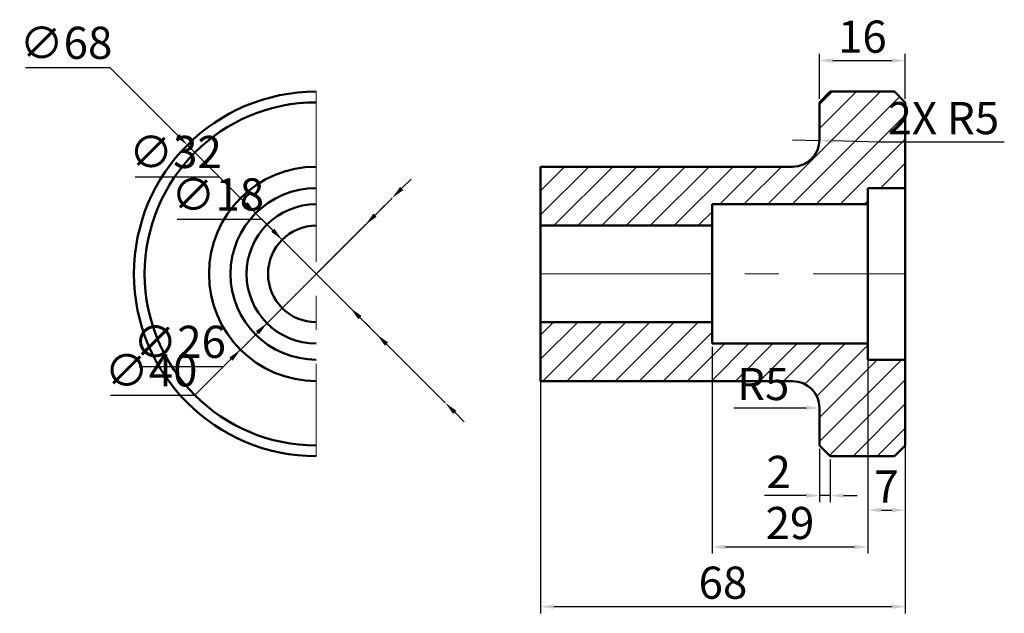
# Model space of a CAD drawing. Units: millimetres. Extents: x 43 to 227, y -15 to 96.
import ezdxf

# ---------------------------------------------------------------- set-up
doc = ezdxf.new("R2010")
doc.units = ezdxf.units.MM
doc.linetypes.add('CENTER', pattern=[50.8, 31.75, -6.35, 6.35, -6.35])
for name, color, linetype, lineweight in [('M-CNTR', 1, 'CENTER', 18), ('M-DIMS', 2, 'Continuous', 25), ('M-HATC', 8, 'Continuous', 18), ('M-OUTL', 7, 'Continuous', 50)]:
    doc.layers.add(name, color=color, linetype=linetype, lineweight=lineweight)
doc.styles.get("Standard").update_dxf_attribs({"font": 'arial.ttf'})
doc.dimstyles.new('ISO-25', dxfattribs={"dimtxt": 6, "dimasz": 2.5, "dimexe": 1.25, "dimexo": 0.625, "dimtad": 1, "dimtoh": 1, "dimdec": 0, "dimtxsty": 'Standard', "dimcen": 2.5, "dimadec": 0, "dimazin": 0, "dimtfac": 1, "dimtdec": 0, "dimtmove": 0, "dimatfit": 3, "dimfxl": 1, "dimarcsym": 0})

# ---------------------------------------------------------------- blocks, each defined once
blk = doc.blocks.new('*D1')
at = {"layer": 'Defpoints', "color": 0, "transparency": 16777216}
for p in [(172.49, 35.65), (201.49, 35.65), (201.49, -2.28)]:
    blk.add_point(p, dxfattribs=at)
at = {"layer": 'M-DIMS', "color": 0, "lineweight": -2, "transparency": 16777216}
for p, q in [((172.49, 35.03), (172.49, -3.53)), ((201.49, 35.03), (201.49, -3.53)), ((174.99, -2.28), (198.99, -2.28))]:
    blk.add_line(p, q, dxfattribs=at)
at = {"layer": 'M-DIMS', "color": 0, "transparency": 16777216}
for points in [[(174.99, -1.87), (174.99, -2.7), (172.49, -2.28)], [(198.99, -1.87), (198.99, -2.7), (201.49, -2.28)]]:
    blk.add_solid(points, dxfattribs=at)
at = {"layer": 'M-DIMS', "color": 0, "transparency": 16777216, "insert": (186.99, 1.41), "char_height": 6, "attachment_point": 5}
blk.add_mtext('29', dxfattribs=at)
blk = doc.blocks.new('*D2')
at = {"layer": 'Defpoints', "color": 0, "transparency": 16777216}
for p in [(140.49, 48.65), (208.49, 48.65), (208.49, -13.41)]:
    blk.add_point(p, dxfattribs=at)
at = {"layer": 'M-DIMS', "color": 0, "lineweight": -2, "transparency": 16777216}
for p, q in [((140.49, 48.03), (140.49, -14.66)), ((208.49, 48.03), (208.49, -14.66)), ((142.99, -13.41), (205.99, -13.41))]:
    blk.add_line(p, q, dxfattribs=at)
at = {"layer": 'M-DIMS', "color": 0, "transparency": 16777216}
for points in [[(142.99, -12.99), (142.99, -13.82), (140.49, -13.41)], [(205.99, -12.99), (205.99, -13.82), (208.49, -13.41)]]:
    blk.add_solid(points, dxfattribs=at)
at = {"layer": 'M-DIMS', "color": 0, "transparency": 16777216, "insert": (174.49, -9.72), "char_height": 6, "attachment_point": 5}
blk.add_mtext('68', dxfattribs=at)
blk = doc.blocks.new('*D3')
at = {"layer": 'Defpoints', "color": 0, "transparency": 16777216}
for p in [(208.49, 88.44), (192.49, 80.65), (208.49, 80.65)]:
    blk.add_point(p, dxfattribs=at)
at = {"layer": 'M-DIMS', "color": 0, "lineweight": -2, "transparency": 16777216}
for p, q in [((192.49, 81.28), (192.49, 89.69)), ((194.99, 88.44), (205.99, 88.44)), ((208.49, 81.28), (208.49, 89.69))]:
    blk.add_line(p, q, dxfattribs=at)
at = {"layer": 'M-DIMS', "color": 0, "transparency": 16777216}
for points in [[(194.99, 88.86), (194.99, 88.03), (192.49, 88.44)], [(205.99, 88.86), (205.99, 88.03), (208.49, 88.44)]]:
    blk.add_solid(points, dxfattribs=at)
at = {"layer": 'M-DIMS', "color": 0, "transparency": 16777216, "insert": (200.49, 92.13), "char_height": 6, "attachment_point": 5}
blk.add_mtext('16', dxfattribs=at)
blk = doc.blocks.new('*D4')
at = {"layer": 'Defpoints', "color": 0, "transparency": 16777216}
for p in [(187.49, 23.65), (192.49, 23.65)]:
    blk.add_point(p, dxfattribs=at)
at = {"layer": 'M-DIMS', "color": 0, "lineweight": -2, "transparency": 16777216}
blk.add_line((176.52, 23.65), (189.99, 23.65), dxfattribs=at)
at = {"layer": 'M-DIMS', "color": 0, "transparency": 16777216}
blk.add_solid([(189.99, 24.07), (189.99, 23.24), (192.49, 23.65)], dxfattribs=at)
at = {"layer": 'M-DIMS', "color": 0, "transparency": 16777216, "insert": (182, 27.33), "char_height": 6, "attachment_point": 5}
blk.add_mtext('R5', dxfattribs=at)
blk = doc.blocks.new('*D5')
at = {"layer": 'Defpoints', "color": 0, "transparency": 16777216}
for p in [(201.49, 32.65), (208.49, 32.65), (208.49, 4.6)]:
    blk.add_point(p, dxfattribs=at)
at = {"layer": 'M-DIMS', "color": 0, "lineweight": -2, "transparency": 16777216}
for p, q in [((201.49, 32.03), (201.49, 3.35)), ((208.49, 32.03), (208.49, 3.35)), ((203.99, 4.6), (205.99, 4.6))]:
    blk.add_line(p, q, dxfattribs=at)
at = {"layer": 'M-DIMS', "color": 0, "transparency": 16777216}
for points in [[(203.99, 5.01), (203.99, 4.18), (201.49, 4.6)], [(205.99, 5.01), (205.99, 4.18), (208.49, 4.6)]]:
    blk.add_solid(points, dxfattribs=at)
at = {"layer": 'M-DIMS', "color": 0, "transparency": 16777216, "insert": (204.99, 8.22), "char_height": 6, "attachment_point": 5}
blk.add_mtext('7', dxfattribs=at)
blk = doc.blocks.new('*D6')
at = {"layer": 'Defpoints', "color": 0, "transparency": 16777216}
for p in [(192.49, 16.65), (194.49, 14.65), (192.49, 7.3)]:
    blk.add_point(p, dxfattribs=at)
at = {"layer": 'M-DIMS', "color": 0, "lineweight": -2, "transparency": 16777216}
for p, q in [((192.49, 16.03), (192.49, 6.05)), ((194.49, 14.03), (194.49, 6.05)), ((189.99, 7.3), (182.26, 7.3)), ((194.49, 7.3), (192.49, 7.3)), ((196.99, 7.3), (199.49, 7.3))]:
    blk.add_line(p, q, dxfattribs=at)
at = {"layer": 'M-DIMS', "color": 0, "transparency": 16777216}
for points in [[(189.99, 7.72), (189.99, 6.89), (192.49, 7.3)], [(196.99, 7.72), (196.99, 6.89), (194.49, 7.3)]]:
    blk.add_solid(points, dxfattribs=at)
at = {"layer": 'M-DIMS', "color": 0, "transparency": 16777216, "insert": (184.88, 10.94), "char_height": 6, "attachment_point": 5}
blk.add_mtext('2', dxfattribs=at)
blk = doc.blocks.new('*D7')
at = {"layer": 'Defpoints', "color": 0, "transparency": 16777216}
for p in [(74.64, 72.69), (122.72, 24.61)]:
    blk.add_point(p, dxfattribs=at)
at = {"layer": 'M-DIMS', "color": 0, "lineweight": -2, "transparency": 16777216}
for p, q in [((44.45, 87.12), (60.21, 87.12)), ((60.21, 87.12), (72.87, 74.46)), ((122.72, 24.61), (74.64, 72.69)), ((124.49, 22.85), (126.26, 21.08))]:
    blk.add_line(p, q, dxfattribs=at)
at = {"layer": 'M-DIMS', "color": 0, "transparency": 16777216}
for points in [[(73.16, 74.76), (72.57, 74.17), (74.64, 72.69)], [(124.79, 23.14), (124.2, 22.55), (122.72, 24.61)]]:
    blk.add_solid(points, dxfattribs=at)
at = {"layer": 'M-DIMS', "color": 0, "transparency": 16777216, "insert": (52.02, 90.97), "char_height": 6, "attachment_point": 5}
blk.add_mtext('∅68', dxfattribs=at)
blk = doc.blocks.new('*D8')
at = {"layer": 'Defpoints', "color": 0, "transparency": 16777216}
for p in [(112.82, 62.8), (84.54, 34.51)]:
    blk.add_point(p, dxfattribs=at)
at = {"layer": 'M-DIMS', "color": 0, "lineweight": -2, "transparency": 16777216}
for p, q in [((114.59, 64.57), (116.36, 66.33)), ((112.82, 62.8), (84.54, 34.51)), ((76.06, 26.02), (82.77, 32.74)), ((60.33, 26.02), (76.06, 26.02))]:
    blk.add_line(p, q, dxfattribs=at)
at = {"layer": 'M-DIMS', "color": 0, "transparency": 16777216}
for points in [[(114.29, 64.86), (114.88, 64.27), (112.82, 62.8)], [(82.48, 33.04), (83.07, 32.45), (84.54, 34.51)]]:
    blk.add_solid(points, dxfattribs=at)
at = {"layer": 'M-DIMS', "color": 0, "transparency": 16777216, "insert": (67.88, 29.88), "char_height": 6, "attachment_point": 5}
blk.add_mtext('∅40', dxfattribs=at)
blk = doc.blocks.new('*D9')
at = {"layer": 'Defpoints', "color": 0, "transparency": 16777216}
for p in [(87.37, 59.97), (109.99, 37.34)]:
    blk.add_point(p, dxfattribs=at)
at = {"layer": 'M-DIMS', "color": 0, "lineweight": -2, "transparency": 16777216}
for p, q in [((64.9, 66.76), (80.58, 66.76)), ((80.58, 66.76), (85.6, 61.74)), ((109.99, 37.34), (87.37, 59.97)), ((111.76, 35.57), (113.53, 33.8))]:
    blk.add_line(p, q, dxfattribs=at)
at = {"layer": 'M-DIMS', "color": 0, "transparency": 16777216}
for points in [[(85.9, 62.03), (85.31, 61.44), (87.37, 59.97)], [(112.05, 35.86), (111.46, 35.28), (109.99, 37.34)]]:
    blk.add_solid(points, dxfattribs=at)
at = {"layer": 'M-DIMS', "color": 0, "transparency": 16777216, "insert": (72.43, 70.62), "char_height": 6, "attachment_point": 5}
blk.add_mtext('∅32', dxfattribs=at)
blk = doc.blocks.new('*D10')
at = {"layer": 'Defpoints', "color": 0, "transparency": 16777216}
for p in [(107.87, 57.85), (89.49, 39.46)]:
    blk.add_point(p, dxfattribs=at)
at = {"layer": 'M-DIMS', "color": 0, "lineweight": -2, "transparency": 16777216}
for p, q in [((109.64, 59.62), (111.41, 61.38)), ((107.87, 57.85), (89.49, 39.46)), ((81.39, 31.35), (87.72, 37.69)), ((65.64, 31.35), (81.39, 31.35))]:
    blk.add_line(p, q, dxfattribs=at)
at = {"layer": 'M-DIMS', "color": 0, "transparency": 16777216}
for points in [[(109.34, 59.91), (109.93, 59.32), (107.87, 57.85)], [(87.43, 37.99), (88.02, 37.4), (89.49, 39.46)]]:
    blk.add_solid(points, dxfattribs=at)
at = {"layer": 'M-DIMS', "color": 0, "transparency": 16777216, "insert": (73.2, 35.21), "char_height": 6, "attachment_point": 5}
blk.add_mtext('∅26', dxfattribs=at)
blk = doc.blocks.new('*D11')
at = {"layer": 'Defpoints', "color": 0, "transparency": 16777216}
for p in [(92.32, 55.02), (105.04, 42.29)]:
    blk.add_point(p, dxfattribs=at)
at = {"layer": 'M-DIMS', "color": 0, "lineweight": -2, "transparency": 16777216}
for p, q in [((72.74, 58.84), (88.5, 58.84)), ((88.5, 58.84), (90.55, 56.79)), ((105.04, 42.29), (92.32, 55.02)), ((106.81, 40.52), (108.58, 38.75))]:
    blk.add_line(p, q, dxfattribs=at)
at = {"layer": 'M-DIMS', "color": 0, "transparency": 16777216}
for points in [[(90.85, 57.08), (90.26, 56.49), (92.32, 55.02)], [(107.1, 40.81), (106.51, 40.22), (105.04, 42.29)]]:
    blk.add_solid(points, dxfattribs=at)
at = {"layer": 'M-DIMS', "color": 0, "transparency": 16777216, "insert": (80.31, 62.7), "char_height": 6, "attachment_point": 5}
blk.add_mtext('∅18', dxfattribs=at)
blk = doc.blocks.new('*D12')
at = {"layer": 'Defpoints', "color": 0, "transparency": 16777216}
for p in [(187.49, 73.65), (192.49, 73.53)]:
    blk.add_point(p, dxfattribs=at)
at = {"layer": 'M-DIMS', "color": 0, "lineweight": -2, "transparency": 16777216}
for p, q in [((187.49, 73.65), (192.49, 73.53)), ((203.61, 73.24), (194.99, 73.46)), ((226.95, 73.24), (203.61, 73.24))]:
    blk.add_line(p, q, dxfattribs=at)
at = {"layer": 'M-DIMS', "color": 0, "transparency": 16777216}
blk.add_solid([(195, 73.88), (194.98, 73.05), (192.49, 73.53)], dxfattribs=at)
at = {"layer": 'M-DIMS', "color": 0, "transparency": 16777216, "insert": (215.59, 76.93), "char_height": 6, "attachment_point": 5}
blk.add_mtext('2X R5', dxfattribs=at)

msp = doc.modelspace()

# ---------------------------------------------------------------- hatches: boundary and pattern name
at = {"layer": 'M-HATC'}
h = msp.add_hatch(dxfattribs=at)
h.set_pattern_fill('ANSI31', color=256)
h.paths.add_polyline_path([(201.49, 64.65), (208.49, 64.65), (208.49, 80.65), (206.49, 82.65), (194.49, 82.65), (192.49, 80.65), (192.49, 73.65, -0.414214), (187.49, 68.65), (140.49, 68.65), (140.49, 57.65), (172.49, 57.65), (172.49, 61.65), (201.49, 61.65)])
h.paths.add_polyline_path([(208.49, 32.65), (201.49, 32.65), (201.49, 35.65), (179.49, 35.65), (172.49, 35.65), (172.49, 39.65), (140.49, 39.65), (140.49, 28.65), (187.49, 28.65, -0.414214), (192.49, 23.65), (192.49, 16.65), (194.49, 14.65), (206.49, 14.65), (208.49, 16.65)])

# ---------------------------------------------------------------- linework, layer by layer
at = {"layer": 'M-CNTR'}
for p, q in [((98.68, 82.65), (98.68, 14.65)), ((140.49, 48.65), (208.49, 48.65))]:
    msp.add_line(p, q, dxfattribs=at)
at = {"layer": 'M-OUTL'}
for p, q in [((192.49, 80.65), (194.49, 82.65)), ((194.49, 82.65), (206.49, 82.65)), ((206.49, 82.65), (208.49, 80.65)), ((192.49, 73.65), (192.49, 80.65)), ((208.49, 80.65), (208.49, 16.65)), ((140.49, 48.65), (140.49, 68.65)), ((140.49, 48.65), (140.49, 68.65)), ((140.49, 68.65), (187.49, 68.65)), ((201.49, 64.65), (208.49, 64.65)), ((201.49, 64.65), (201.49, 32.65)), ((172.49, 61.65), (201.49, 61.65)), ((172.49, 48.65), (172.49, 61.65)), ((140.49, 57.65), (172.49, 57.65)), ((140.49, 48.65), (140.49, 28.65)), ((172.49, 48.65), (172.49, 35.65)), ((140.49, 39.65), (172.49, 39.65)), ((179.49, 35.65), (172.49, 35.65)), ((179.49, 35.65), (201.49, 35.65)), ((201.49, 32.65), (208.49, 32.65)), ((140.49, 28.65), (187.49, 28.65)), ((192.49, 23.65), (192.49, 16.65)), ((192.49, 16.65), (194.49, 14.65)), ((208.49, 16.65), (206.49, 14.65)), ((206.49, 14.65), (194.49, 14.65))]:
    msp.add_line(p, q, dxfattribs=at)
for centre, radius, start, end in [((98.68, 48.65), 34, 90, 270), ((98.68, 48.65), 32, 90, 270), ((98.68, 48.65), 32, 90, 270), ((187.49, 73.65), 5, 270, 0), ((98.68, 48.65), 20, 90, 270), ((98.68, 48.65), 16, 90, 270), ((98.68, 48.65), 13, 90, 270), ((98.68, 48.65), 9, 90, 270), ((187.49, 23.65), 5, 0, 90)]:
    msp.add_arc(centre, radius, start, end, dxfattribs=at)

# ---------------------------------------------------------------- dimensions: what is measured, and where the dimension line sits
at = {"layer": 'M-DIMS'}
for base, p1, p2, override, picture, middle in [((208.49, 88.44), (192.49, 80.65), (208.49, 80.65), {"dimclrd": 0, "dimclre": 0, "dimclrt": 0}, '*D3', (200.49, 92.13)), ((208.49, -13.41), (140.49, 48.65), (208.49, 48.65), {"dimclrd": 0, "dimclre": 0, "dimclrt": 0}, '*D2', (174.49, -9.72)), ((201.49, -2.28), (172.49, 35.65), (201.49, 35.65), {"dimclrd": 0, "dimclre": 0, "dimclrt": 0}, '*D1', (186.99, 1.41)), ((208.49, 4.6), (201.49, 32.65), (208.49, 32.65), {"dimclrd": 0, "dimclre": 0, "dimclrt": 0}, '*D5', (204.99, 8.22)), ((192.49, 7.3), (194.49, 14.65), (192.49, 16.65), {"dimdec": 0, "dimlfac": 1, "dimrnd": 0, "dimzin": 0, "dimdsep": 46, "dimlunit": 2}, '*D6', (184.88, 10.94))]:
    dim = msp.add_linear_dim(base=base, p1=p1, p2=p2, dimstyle='ISO-25', override=override, dxfattribs=at)
    dim.commit()
    dim.dimension.update_dxf_attribs({"geometry": picture, "text_midpoint": middle})
for p1, p2, picture, middle in [((122.72, 24.61), (74.64, 72.69), '*D7', (52.02, 87.12)), ((109.99, 37.34), (87.37, 59.97), '*D9', (72.43, 66.76)), ((112.82, 62.8), (84.54, 34.51), '*D8', (67.88, 26.02)), ((105.04, 42.29), (92.32, 55.02), '*D11', (80.31, 58.84)), ((107.87, 57.85), (89.49, 39.46), '*D10', (73.2, 31.35))]:
    dim = msp.add_diameter_dim_2p(p1=p1, p2=p2, dimstyle='ISO-25', override={"dimdec": 0, "dimlfac": 1, "dimrnd": 0, "dimzin": 0, "dimdsep": 46, "dimlunit": 2}, dxfattribs=at)
    dim.commit()
    dim.dimension.update_dxf_attribs({"geometry": picture, "text_midpoint": middle, "dimtype": 163})
dim = msp.add_radius_dim(center=(187.49, 73.65), mpoint=(192.49, 73.53), text='2X <>', dimstyle='ISO-25', override={"dimdec": 0, "dimlfac": 1, "dimrnd": 0, "dimzin": 0, "dimdsep": 46, "dimlunit": 2}, dxfattribs=at)
dim.commit()
dim.dimension.update_dxf_attribs({"geometry": '*D12', "text_midpoint": (215.59, 76.93)})
dim = msp.add_radius_dim(center=(187.49, 23.65), mpoint=(192.49, 23.65), dimstyle='ISO-25', override={"dimclrd": 0, "dimclre": 0, "dimclrt": 0}, dxfattribs=at)
dim.commit()
dim.dimension.update_dxf_attribs({"geometry": '*D4', "text_midpoint": (182, 23.65), "dimtype": 164})

doc.saveas('drawing.dxf')
